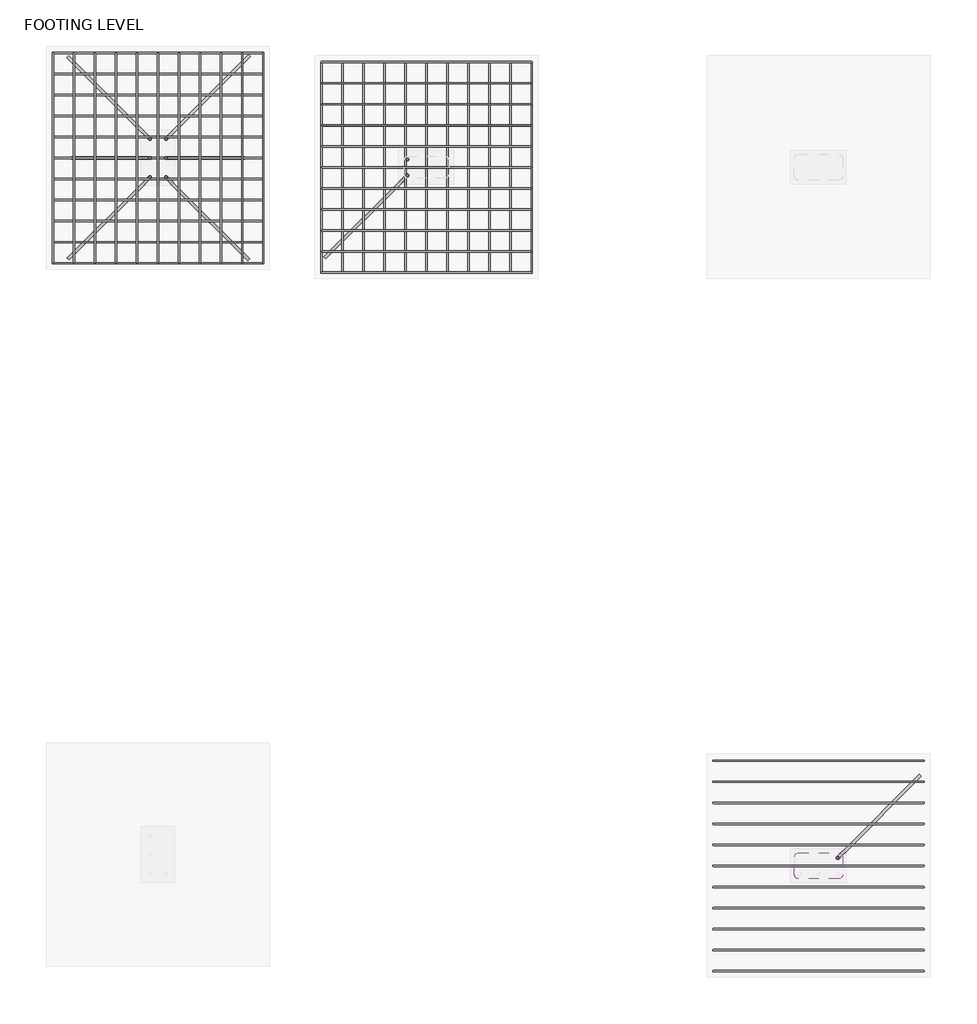
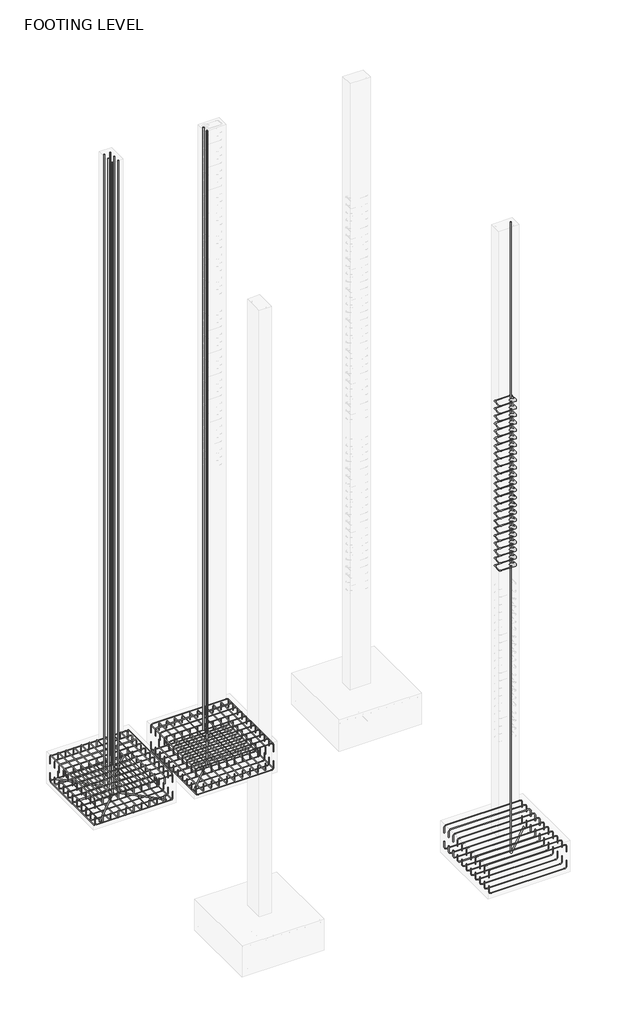
# One storey, part 3 of 10: 24 reinforcing bars.
"""IFC4 building model written with IfcOpenShell, lengths in millimetres."""

from ifc_helpers import new_model, si_unit, point, frame, origin, place, context, project, spatial, polyline, circle_curve, trimmed, segment, composite_curve, source, transform, mapped, element, save
from ifc_brep_helpers import swept_disk

model = new_model("IFC4")

# Units and contexts
model_context = context("Model", 3, world=origin())
ifc_project = project(units=[si_unit("LENGTHUNIT", "METRE", prefix="MILLI")], contexts=[model_context])

# Site, building, storey
site = spatial("IfcSite", under=ifc_project)
building = spatial("IfcBuilding", under=site)
storey = spatial("IfcBuildingStorey", under=building, Name="FOOTING LEVEL", Elevation=-1371.6)

# Reinforcing bars
placement = place(None, origin())
reinforcing_bar_shape = source(origin(), model_context, "Body", "SolidModel", [
    swept_disk(composite_curve([segment(polyline([(-12158.3043223, 4208.9876382, -1562.1), (-12158.3043223, 4208.9876382, -1447.8)]), True, "CONTINUOUS"), segment(trimmed(circle_curve(frame((-12191.6418223, 4208.9876382, -1447.8), z_axis=(0.0, -1.0, 0.0), x_axis=(33.337499999999636, 0.0, 0.0)), 33.3375), [point((-12158.3043223, 4208.9876382, -1447.8))], [point((-12191.6418223, 4208.9876382, -1414.4625))], True, "CARTESIAN"), True, "CONTINUOUS"), segment(polyline([(-12191.6418223, 4208.9876382, -1414.4625), (-13563.2418223, 4208.9876382, -1414.4625)]), True, "CONTINUOUS"), segment(trimmed(circle_curve(frame((-13563.2418223, 4208.9876382, -1447.8), z_axis=(0.0, -1.0, 0.0), x_axis=(0.0, 0.0, 33.337499999999864)), 33.3375), [point((-13563.2418223, 4208.9876382, -1414.4625))], [point((-13596.5793223, 4208.9876382, -1447.8))], True, "CARTESIAN"), True, "CONTINUOUS"), segment(polyline([(-13596.5793223, 4208.9876382, -1447.8), (-13596.5793223, 4208.9876382, -1562.1)]), True, "CONTINUOUS")], self_intersect=False), 4.7625),
])
element("IfcReinforcingBar", 1, at=placement, inside=storey, context=model_context, shape_type="MappedRepresentation", body=[
    mapped(reinforcing_bar_shape, transform((0.0, 0.0, 0.0), x_axis=(1.0, 0.0, 0.0), y_axis=(0.0, 1.0, 0.0), z_axis=(0.0, 0.0, 1.0))),
    mapped(reinforcing_bar_shape, transform((0.0, 143.8275, 0.0), x_axis=(1.0, 0.0, 0.0), y_axis=(0.0, 1.0, 0.0), z_axis=(0.0, 0.0, 1.0))),
    mapped(reinforcing_bar_shape, transform((0.0, 287.655, 0.0), x_axis=(1.0, 0.0, 0.0), y_axis=(0.0, 1.0, 0.0), z_axis=(0.0, 0.0, 1.0))),
    mapped(reinforcing_bar_shape, transform((0.0, 431.4825, 0.0), x_axis=(1.0, 0.0, 0.0), y_axis=(0.0, 1.0, 0.0), z_axis=(0.0, 0.0, 1.0))),
    mapped(reinforcing_bar_shape, transform((0.0, 575.31, 0.0), x_axis=(1.0, 0.0, 0.0), y_axis=(0.0, 1.0, 0.0), z_axis=(0.0, 0.0, 1.0))),
    mapped(reinforcing_bar_shape, transform((0.0, 719.1375, 0.0), x_axis=(1.0, 0.0, 0.0), y_axis=(0.0, 1.0, 0.0), z_axis=(0.0, 0.0, 1.0))),
    mapped(reinforcing_bar_shape, transform((0.0, 862.965, 0.0), x_axis=(1.0, 0.0, 0.0), y_axis=(0.0, 1.0, 0.0), z_axis=(0.0, 0.0, 1.0))),
    mapped(reinforcing_bar_shape, transform((0.0, 1006.7925, 0.0), x_axis=(1.0, 0.0, 0.0), y_axis=(0.0, 1.0, 0.0), z_axis=(0.0, 0.0, 1.0))),
    mapped(reinforcing_bar_shape, transform((0.0, 1150.62, 0.0), x_axis=(1.0, 0.0, 0.0), y_axis=(0.0, 1.0, 0.0), z_axis=(0.0, 0.0, 1.0))),
    mapped(reinforcing_bar_shape, transform((0.0, 1294.4475, 0.0), x_axis=(1.0, 0.0, 0.0), y_axis=(0.0, 1.0, 0.0), z_axis=(0.0, 0.0, 1.0))),
    mapped(reinforcing_bar_shape, transform((0.0, 1438.275, 0.0), x_axis=(1.0, 0.0, 0.0), y_axis=(0.0, 1.0, 0.0), z_axis=(0.0, 0.0, 1.0))),
])
reinforcing_bar_2_shape = source(origin(), model_context, "Body", "SolidModel", [
    swept_disk(composite_curve([segment(polyline([(-13596.5793223, 4208.9876382, -1790.7), (-13596.5793223, 4208.9876382, -1905.0)]), True, "CONTINUOUS"), segment(trimmed(circle_curve(frame((-13563.2418223, 4208.9876382, -1905.0), z_axis=(0.0, -1.0, 0.0), x_axis=(-33.337499999999636, 0.0, 0.0)), 33.3375), [point((-13596.5793223, 4208.9876382, -1905.0))], [point((-13563.2418223, 4208.9876382, -1938.3375))], True, "CARTESIAN"), True, "CONTINUOUS"), segment(polyline([(-13563.2418223, 4208.9876382, -1938.3375), (-12191.6418223, 4208.9876382, -1938.3375)]), True, "CONTINUOUS"), segment(trimmed(circle_curve(frame((-12191.6418223, 4208.9876382, -1905.0), z_axis=(0.0, -1.0, 0.0), x_axis=(0.0, 0.0, -33.33750000000009)), 33.3375), [point((-12191.6418223, 4208.9876382, -1938.3375))], [point((-12158.3043223, 4208.9876382, -1905.0))], True, "CARTESIAN"), True, "CONTINUOUS"), segment(polyline([(-12158.3043223, 4208.9876382, -1905.0), (-12158.3043223, 4208.9876382, -1790.7)]), True, "CONTINUOUS")], self_intersect=False), 4.7625),
])
element("IfcReinforcingBar", 2, at=placement, inside=storey, context=model_context, shape_type="MappedRepresentation", body=[
    mapped(reinforcing_bar_2_shape, transform((0.0, 0.0, 0.0), x_axis=(1.0, 0.0, 0.0), y_axis=(0.0, 1.0, 0.0), z_axis=(0.0, 0.0, 1.0))),
    mapped(reinforcing_bar_2_shape, transform((0.0, 143.8275, 0.0), x_axis=(1.0, 0.0, 0.0), y_axis=(0.0, 1.0, 0.0), z_axis=(0.0, 0.0, 1.0))),
    mapped(reinforcing_bar_2_shape, transform((0.0, 287.655, 0.0), x_axis=(1.0, 0.0, 0.0), y_axis=(0.0, 1.0, 0.0), z_axis=(0.0, 0.0, 1.0))),
    mapped(reinforcing_bar_2_shape, transform((0.0, 431.4825, 0.0), x_axis=(1.0, 0.0, 0.0), y_axis=(0.0, 1.0, 0.0), z_axis=(0.0, 0.0, 1.0))),
    mapped(reinforcing_bar_2_shape, transform((0.0, 575.31, 0.0), x_axis=(1.0, 0.0, 0.0), y_axis=(0.0, 1.0, 0.0), z_axis=(0.0, 0.0, 1.0))),
    mapped(reinforcing_bar_2_shape, transform((0.0, 719.1375, 0.0), x_axis=(1.0, 0.0, 0.0), y_axis=(0.0, 1.0, 0.0), z_axis=(0.0, 0.0, 1.0))),
    mapped(reinforcing_bar_2_shape, transform((0.0, 862.965, 0.0), x_axis=(1.0, 0.0, 0.0), y_axis=(0.0, 1.0, 0.0), z_axis=(0.0, 0.0, 1.0))),
    mapped(reinforcing_bar_2_shape, transform((0.0, 1006.7925, 0.0), x_axis=(1.0, 0.0, 0.0), y_axis=(0.0, 1.0, 0.0), z_axis=(0.0, 0.0, 1.0))),
    mapped(reinforcing_bar_2_shape, transform((0.0, 1150.62, 0.0), x_axis=(1.0, 0.0, 0.0), y_axis=(0.0, 1.0, 0.0), z_axis=(0.0, 0.0, 1.0))),
    mapped(reinforcing_bar_2_shape, transform((0.0, 1294.4475, 0.0), x_axis=(1.0, 0.0, 0.0), y_axis=(0.0, 1.0, 0.0), z_axis=(0.0, 0.0, 1.0))),
    mapped(reinforcing_bar_2_shape, transform((0.0, 1438.275, 0.0), x_axis=(1.0, 0.0, 0.0), y_axis=(0.0, 1.0, 0.0), z_axis=(0.0, 0.0, 1.0))),
])
reinforcing_bar_3_shape = source(origin(), model_context, "Body", "SolidModel", [
    swept_disk(composite_curve([segment(polyline([(-13596.5793223, 5647.2626382, -1770.864029), (-13596.5793223, 5647.2626382, -1885.164029)]), True, "CONTINUOUS"), segment(trimmed(circle_curve(frame((-13596.5793223, 5613.9251382, -1885.164029), z_axis=(-1.0, 0.0, 0.0), x_axis=(0.0, 33.337499999999636, 0.0)), 33.3375), [point((-13596.5793223, 5647.2626382, -1885.164029))], [point((-13596.5793223, 5613.9251382, -1918.501529))], True, "CARTESIAN"), True, "CONTINUOUS"), segment(polyline([(-13596.5793223, 5613.9251382, -1918.501529), (-13596.5793223, 4242.3251382, -1918.501529)]), True, "CONTINUOUS"), segment(trimmed(circle_curve(frame((-13596.5793223, 4242.3251382, -1885.164029), z_axis=(-1.0, 0.0, 0.0), x_axis=(0.0, 0.0, -33.337499999999864)), 33.3375), [point((-13596.5793223, 4242.3251382, -1918.501529))], [point((-13596.5793223, 4208.9876382, -1885.164029))], True, "CARTESIAN"), True, "CONTINUOUS"), segment(polyline([(-13596.5793223, 4208.9876382, -1885.164029), (-13596.5793223, 4208.9876382, -1770.864029)]), True, "CONTINUOUS")], self_intersect=False), 4.7625),
])
element("IfcReinforcingBar", 3, at=placement, inside=storey, context=model_context, shape_type="MappedRepresentation", body=[
    mapped(reinforcing_bar_3_shape, transform((0.0, 0.0, 0.0), x_axis=(1.0, 0.0, 0.0), y_axis=(0.0, 1.0, 0.0), z_axis=(0.0, 0.0, 1.0))),
    mapped(reinforcing_bar_3_shape, transform((143.8275, 0.0, 0.0), x_axis=(1.0, 0.0, 0.0), y_axis=(0.0, 1.0, 0.0), z_axis=(0.0, 0.0, 1.0))),
    mapped(reinforcing_bar_3_shape, transform((287.655, 0.0, 0.0), x_axis=(1.0, 0.0, 0.0), y_axis=(0.0, 1.0, 0.0), z_axis=(0.0, 0.0, 1.0))),
    mapped(reinforcing_bar_3_shape, transform((431.4825, 0.0, 0.0), x_axis=(1.0, 0.0, 0.0), y_axis=(0.0, 1.0, 0.0), z_axis=(0.0, 0.0, 1.0))),
    mapped(reinforcing_bar_3_shape, transform((575.31, 0.0, 0.0), x_axis=(1.0, 0.0, 0.0), y_axis=(0.0, 1.0, 0.0), z_axis=(0.0, 0.0, 1.0))),
    mapped(reinforcing_bar_3_shape, transform((719.1375, 0.0, 0.0), x_axis=(1.0, 0.0, 0.0), y_axis=(0.0, 1.0, 0.0), z_axis=(0.0, 0.0, 1.0))),
    mapped(reinforcing_bar_3_shape, transform((862.965, 0.0, 0.0), x_axis=(1.0, 0.0, 0.0), y_axis=(0.0, 1.0, 0.0), z_axis=(0.0, 0.0, 1.0))),
    mapped(reinforcing_bar_3_shape, transform((1006.7925, 0.0, 0.0), x_axis=(1.0, 0.0, 0.0), y_axis=(0.0, 1.0, 0.0), z_axis=(0.0, 0.0, 1.0))),
    mapped(reinforcing_bar_3_shape, transform((1150.62, 0.0, 0.0), x_axis=(1.0, 0.0, 0.0), y_axis=(0.0, 1.0, 0.0), z_axis=(0.0, 0.0, 1.0))),
    mapped(reinforcing_bar_3_shape, transform((1294.4475, 0.0, 0.0), x_axis=(1.0, 0.0, 0.0), y_axis=(0.0, 1.0, 0.0), z_axis=(0.0, 0.0, 1.0))),
    mapped(reinforcing_bar_3_shape, transform((1438.275, 0.0, 0.0), x_axis=(1.0, 0.0, 0.0), y_axis=(0.0, 1.0, 0.0), z_axis=(0.0, 0.0, 1.0))),
])
reinforcing_bar_4_shape = source(origin(), model_context, "Body", "SolidModel", [
    swept_disk(composite_curve([segment(polyline([(-12158.3043223, 5647.2626382, -1586.5406765), (-12158.3043223, 5647.2626382, -1472.2406765)]), True, "CONTINUOUS"), segment(trimmed(circle_curve(frame((-12158.3043223, 5613.9251382, -1472.2406765), z_axis=(1.0, 0.0, 0.0), x_axis=(0.0, 33.337499999999636, 0.0)), 33.3375), [point((-12158.3043223, 5647.2626382, -1472.2406765))], [point((-12158.3043223, 5613.9251382, -1438.9031765))], True, "CARTESIAN"), True, "CONTINUOUS"), segment(polyline([(-12158.3043223, 5613.9251382, -1438.9031765), (-12158.3043223, 4242.3251382, -1438.9031765)]), True, "CONTINUOUS"), segment(trimmed(circle_curve(frame((-12158.3043223, 4242.3251382, -1472.2406765), z_axis=(1.0, 0.0, 0.0), x_axis=(0.0, 0.0, 33.33750000000009)), 33.3375), [point((-12158.3043223, 4242.3251382, -1438.9031765))], [point((-12158.3043223, 4208.9876382, -1472.2406765))], True, "CARTESIAN"), True, "CONTINUOUS"), segment(polyline([(-12158.3043223, 4208.9876382, -1472.2406765), (-12158.3043223, 4208.9876382, -1586.5406765)]), True, "CONTINUOUS")], self_intersect=False), 4.7625),
])
element("IfcReinforcingBar", 4, at=placement, inside=storey, context=model_context, shape_type="MappedRepresentation", body=[
    mapped(reinforcing_bar_4_shape, transform((0.0, 0.0, 0.0), x_axis=(1.0, 0.0, 0.0), y_axis=(0.0, 1.0, 0.0), z_axis=(0.0, 0.0, 1.0))),
    mapped(reinforcing_bar_4_shape, transform((-143.8275, 0.0, 0.0), x_axis=(1.0, 0.0, 0.0), y_axis=(0.0, 1.0, 0.0), z_axis=(0.0, 0.0, 1.0))),
    mapped(reinforcing_bar_4_shape, transform((-287.655, 0.0, 0.0), x_axis=(1.0, 0.0, 0.0), y_axis=(0.0, 1.0, 0.0), z_axis=(0.0, 0.0, 1.0))),
    mapped(reinforcing_bar_4_shape, transform((-431.4825, 0.0, 0.0), x_axis=(1.0, 0.0, 0.0), y_axis=(0.0, 1.0, 0.0), z_axis=(0.0, 0.0, 1.0))),
    mapped(reinforcing_bar_4_shape, transform((-575.31, 0.0, 0.0), x_axis=(1.0, 0.0, 0.0), y_axis=(0.0, 1.0, 0.0), z_axis=(0.0, 0.0, 1.0))),
    mapped(reinforcing_bar_4_shape, transform((-719.1375, 0.0, 0.0), x_axis=(1.0, 0.0, 0.0), y_axis=(0.0, 1.0, 0.0), z_axis=(0.0, 0.0, 1.0))),
    mapped(reinforcing_bar_4_shape, transform((-862.965, 0.0, 0.0), x_axis=(1.0, 0.0, 0.0), y_axis=(0.0, 1.0, 0.0), z_axis=(0.0, 0.0, 1.0))),
    mapped(reinforcing_bar_4_shape, transform((-1006.7925, 0.0, 0.0), x_axis=(1.0, 0.0, 0.0), y_axis=(0.0, 1.0, 0.0), z_axis=(0.0, 0.0, 1.0))),
    mapped(reinforcing_bar_4_shape, transform((-1150.62, 0.0, 0.0), x_axis=(1.0, 0.0, 0.0), y_axis=(0.0, 1.0, 0.0), z_axis=(0.0, 0.0, 1.0))),
    mapped(reinforcing_bar_4_shape, transform((-1294.4475, 0.0, 0.0), x_axis=(1.0, 0.0, 0.0), y_axis=(0.0, 1.0, 0.0), z_axis=(0.0, 0.0, 1.0))),
    mapped(reinforcing_bar_4_shape, transform((-1438.275, 0.0, 0.0), x_axis=(1.0, 0.0, 0.0), y_axis=(0.0, 1.0, 0.0), z_axis=(0.0, 0.0, 1.0))),
])
reinforcing_bar_5_shape = source(origin(), model_context, "Body", "SolidModel", [
    swept_disk(composite_curve([segment(polyline([(-13993.4543223, 5711.1953802, -1562.1), (-13993.4543223, 5711.1953802, -1447.8)]), True, "CONTINUOUS"), segment(trimmed(circle_curve(frame((-13993.4543223, 5677.8578802, -1447.8), z_axis=(1.0, 0.0, 0.0), x_axis=(0.0, 33.337499999999636, 0.0)), 33.3375), [point((-13993.4543223, 5711.1953802, -1447.8))], [point((-13993.4543223, 5677.8578802, -1414.4625))], True, "CARTESIAN"), True, "CONTINUOUS"), segment(polyline([(-13993.4543223, 5677.8578802, -1414.4625), (-13993.4543223, 4306.2578802, -1414.4625)]), True, "CONTINUOUS"), segment(trimmed(circle_curve(frame((-13993.4543223, 4306.2578802, -1447.8), z_axis=(1.0, 0.0, 0.0), x_axis=(0.0, 0.0, 33.337499999999864)), 33.3375), [point((-13993.4543223, 4306.2578802, -1414.4625))], [point((-13993.4543223, 4272.9203802, -1447.8))], True, "CARTESIAN"), True, "CONTINUOUS"), segment(polyline([(-13993.4543223, 4272.9203802, -1447.8), (-13993.4543223, 4272.9203802, -1562.1)]), True, "CONTINUOUS")], self_intersect=False), 4.7625),
])
element("IfcReinforcingBar", 5, at=placement, inside=storey, context=model_context, shape_type="MappedRepresentation", body=[
    mapped(reinforcing_bar_5_shape, transform((0.0, 0.0, 0.0), x_axis=(1.0, 0.0, 0.0), y_axis=(0.0, 1.0, 0.0), z_axis=(0.0, 0.0, 1.0))),
    mapped(reinforcing_bar_5_shape, transform((-143.8275, 0.0, 0.0), x_axis=(1.0, 0.0, 0.0), y_axis=(0.0, 1.0, 0.0), z_axis=(0.0, 0.0, 1.0))),
    mapped(reinforcing_bar_5_shape, transform((-287.655, 0.0, 0.0), x_axis=(1.0, 0.0, 0.0), y_axis=(0.0, 1.0, 0.0), z_axis=(0.0, 0.0, 1.0))),
    mapped(reinforcing_bar_5_shape, transform((-431.4825, 0.0, 0.0), x_axis=(1.0, 0.0, 0.0), y_axis=(0.0, 1.0, 0.0), z_axis=(0.0, 0.0, 1.0))),
    mapped(reinforcing_bar_5_shape, transform((-575.31, 0.0, 0.0), x_axis=(1.0, 0.0, 0.0), y_axis=(0.0, 1.0, 0.0), z_axis=(0.0, 0.0, 1.0))),
    mapped(reinforcing_bar_5_shape, transform((-719.1375, 0.0, 0.0), x_axis=(1.0, 0.0, 0.0), y_axis=(0.0, 1.0, 0.0), z_axis=(0.0, 0.0, 1.0))),
    mapped(reinforcing_bar_5_shape, transform((-862.965, 0.0, 0.0), x_axis=(1.0, 0.0, 0.0), y_axis=(0.0, 1.0, 0.0), z_axis=(0.0, 0.0, 1.0))),
    mapped(reinforcing_bar_5_shape, transform((-1006.7925, 0.0, 0.0), x_axis=(1.0, 0.0, 0.0), y_axis=(0.0, 1.0, 0.0), z_axis=(0.0, 0.0, 1.0))),
    mapped(reinforcing_bar_5_shape, transform((-1150.62, 0.0, 0.0), x_axis=(1.0, 0.0, 0.0), y_axis=(0.0, 1.0, 0.0), z_axis=(0.0, 0.0, 1.0))),
    mapped(reinforcing_bar_5_shape, transform((-1294.4475, 0.0, 0.0), x_axis=(1.0, 0.0, 0.0), y_axis=(0.0, 1.0, 0.0), z_axis=(0.0, 0.0, 1.0))),
    mapped(reinforcing_bar_5_shape, transform((-1438.275, 0.0, 0.0), x_axis=(1.0, 0.0, 0.0), y_axis=(0.0, 1.0, 0.0), z_axis=(0.0, 0.0, 1.0))),
])
reinforcing_bar_6_shape = source(origin(), model_context, "Body", "SolidModel", [
    swept_disk(composite_curve([segment(polyline([(-13993.4543223, 4272.9203802, -1790.7), (-13993.4543223, 4272.9203802, -1905.0)]), True, "CONTINUOUS"), segment(trimmed(circle_curve(frame((-13993.4543223, 4306.2578802, -1905.0), z_axis=(1.0, 0.0, 0.0), x_axis=(0.0, -33.337499999999636, 0.0)), 33.3375), [point((-13993.4543223, 4272.9203802, -1905.0))], [point((-13993.4543223, 4306.2578802, -1938.3375))], True, "CARTESIAN"), True, "CONTINUOUS"), segment(polyline([(-13993.4543223, 4306.2578802, -1938.3375), (-13993.4543223, 5677.8578802, -1938.3375)]), True, "CONTINUOUS"), segment(trimmed(circle_curve(frame((-13993.4543223, 5677.8578802, -1905.0), z_axis=(1.0, 0.0, 0.0), x_axis=(0.0, 0.0, -33.33750000000009)), 33.3375), [point((-13993.4543223, 5677.8578802, -1938.3375))], [point((-13993.4543223, 5711.1953802, -1905.0))], True, "CARTESIAN"), True, "CONTINUOUS"), segment(polyline([(-13993.4543223, 5711.1953802, -1905.0), (-13993.4543223, 5711.1953802, -1790.7)]), True, "CONTINUOUS")], self_intersect=False), 4.7625),
])
element("IfcReinforcingBar", 6, at=placement, inside=storey, context=model_context, shape_type="MappedRepresentation", body=[
    mapped(reinforcing_bar_6_shape, transform((0.0, 0.0, 0.0), x_axis=(1.0, 0.0, 0.0), y_axis=(0.0, 1.0, 0.0), z_axis=(0.0, 0.0, 1.0))),
    mapped(reinforcing_bar_6_shape, transform((-143.8275, 0.0, 0.0), x_axis=(1.0, 0.0, 0.0), y_axis=(0.0, 1.0, 0.0), z_axis=(0.0, 0.0, 1.0))),
    mapped(reinforcing_bar_6_shape, transform((-287.655, 0.0, 0.0), x_axis=(1.0, 0.0, 0.0), y_axis=(0.0, 1.0, 0.0), z_axis=(0.0, 0.0, 1.0))),
    mapped(reinforcing_bar_6_shape, transform((-431.4825, 0.0, 0.0), x_axis=(1.0, 0.0, 0.0), y_axis=(0.0, 1.0, 0.0), z_axis=(0.0, 0.0, 1.0))),
    mapped(reinforcing_bar_6_shape, transform((-575.31, 0.0, 0.0), x_axis=(1.0, 0.0, 0.0), y_axis=(0.0, 1.0, 0.0), z_axis=(0.0, 0.0, 1.0))),
    mapped(reinforcing_bar_6_shape, transform((-719.1375, 0.0, 0.0), x_axis=(1.0, 0.0, 0.0), y_axis=(0.0, 1.0, 0.0), z_axis=(0.0, 0.0, 1.0))),
    mapped(reinforcing_bar_6_shape, transform((-862.965, 0.0, 0.0), x_axis=(1.0, 0.0, 0.0), y_axis=(0.0, 1.0, 0.0), z_axis=(0.0, 0.0, 1.0))),
    mapped(reinforcing_bar_6_shape, transform((-1006.7925, 0.0, 0.0), x_axis=(1.0, 0.0, 0.0), y_axis=(0.0, 1.0, 0.0), z_axis=(0.0, 0.0, 1.0))),
    mapped(reinforcing_bar_6_shape, transform((-1150.62, 0.0, 0.0), x_axis=(1.0, 0.0, 0.0), y_axis=(0.0, 1.0, 0.0), z_axis=(0.0, 0.0, 1.0))),
    mapped(reinforcing_bar_6_shape, transform((-1294.4475, 0.0, 0.0), x_axis=(1.0, 0.0, 0.0), y_axis=(0.0, 1.0, 0.0), z_axis=(0.0, 0.0, 1.0))),
    mapped(reinforcing_bar_6_shape, transform((-1438.275, 0.0, 0.0), x_axis=(1.0, 0.0, 0.0), y_axis=(0.0, 1.0, 0.0), z_axis=(0.0, 0.0, 1.0))),
])
reinforcing_bar_7_shape = source(origin(), model_context, "Body", "SolidModel", [
    swept_disk(composite_curve([segment(polyline([(-15431.7293223, 4272.9203802, -1770.864029), (-15431.7293223, 4272.9203802, -1885.164029)]), True, "CONTINUOUS"), segment(trimmed(circle_curve(frame((-15398.3918223, 4272.9203802, -1885.164029), z_axis=(0.0, -1.0, 0.0), x_axis=(-33.337499999999636, 0.0, 0.0)), 33.3375), [point((-15431.7293223, 4272.9203802, -1885.164029))], [point((-15398.3918223, 4272.9203802, -1918.501529))], True, "CARTESIAN"), True, "CONTINUOUS"), segment(polyline([(-15398.3918223, 4272.9203802, -1918.501529), (-14026.7918223, 4272.9203802, -1918.501529)]), True, "CONTINUOUS"), segment(trimmed(circle_curve(frame((-14026.7918223, 4272.9203802, -1885.164029), z_axis=(0.0, -1.0, 0.0), x_axis=(0.0, 0.0, -33.337499999999864)), 33.3375), [point((-14026.7918223, 4272.9203802, -1918.501529))], [point((-13993.4543223, 4272.9203802, -1885.164029))], True, "CARTESIAN"), True, "CONTINUOUS"), segment(polyline([(-13993.4543223, 4272.9203802, -1885.164029), (-13993.4543223, 4272.9203802, -1770.864029)]), True, "CONTINUOUS")], self_intersect=False), 4.7625),
])
element("IfcReinforcingBar", 7, at=placement, inside=storey, context=model_context, shape_type="MappedRepresentation", body=[
    mapped(reinforcing_bar_7_shape, transform((0.0, 0.0, 0.0), x_axis=(1.0, 0.0, 0.0), y_axis=(0.0, 1.0, 0.0), z_axis=(0.0, 0.0, 1.0))),
    mapped(reinforcing_bar_7_shape, transform((0.0, 143.8275, 0.0), x_axis=(1.0, 0.0, 0.0), y_axis=(0.0, 1.0, 0.0), z_axis=(0.0, 0.0, 1.0))),
    mapped(reinforcing_bar_7_shape, transform((0.0, 287.655, 0.0), x_axis=(1.0, 0.0, 0.0), y_axis=(0.0, 1.0, 0.0), z_axis=(0.0, 0.0, 1.0))),
    mapped(reinforcing_bar_7_shape, transform((0.0, 431.4825, 0.0), x_axis=(1.0, 0.0, 0.0), y_axis=(0.0, 1.0, 0.0), z_axis=(0.0, 0.0, 1.0))),
    mapped(reinforcing_bar_7_shape, transform((0.0, 575.31, 0.0), x_axis=(1.0, 0.0, 0.0), y_axis=(0.0, 1.0, 0.0), z_axis=(0.0, 0.0, 1.0))),
    mapped(reinforcing_bar_7_shape, transform((0.0, 719.1375, 0.0), x_axis=(1.0, 0.0, 0.0), y_axis=(0.0, 1.0, 0.0), z_axis=(0.0, 0.0, 1.0))),
    mapped(reinforcing_bar_7_shape, transform((0.0, 862.965, 0.0), x_axis=(1.0, 0.0, 0.0), y_axis=(0.0, 1.0, 0.0), z_axis=(0.0, 0.0, 1.0))),
    mapped(reinforcing_bar_7_shape, transform((0.0, 1006.7925, 0.0), x_axis=(1.0, 0.0, 0.0), y_axis=(0.0, 1.0, 0.0), z_axis=(0.0, 0.0, 1.0))),
    mapped(reinforcing_bar_7_shape, transform((0.0, 1150.62, 0.0), x_axis=(1.0, 0.0, 0.0), y_axis=(0.0, 1.0, 0.0), z_axis=(0.0, 0.0, 1.0))),
    mapped(reinforcing_bar_7_shape, transform((0.0, 1294.4475, 0.0), x_axis=(1.0, 0.0, 0.0), y_axis=(0.0, 1.0, 0.0), z_axis=(0.0, 0.0, 1.0))),
    mapped(reinforcing_bar_7_shape, transform((0.0, 1438.275, 0.0), x_axis=(1.0, 0.0, 0.0), y_axis=(0.0, 1.0, 0.0), z_axis=(0.0, 0.0, 1.0))),
])
reinforcing_bar_8_shape = source(origin(), model_context, "Body", "SolidModel", [
    swept_disk(composite_curve([segment(polyline([(-15431.7293223, 5711.1953802, -1586.5406765), (-15431.7293223, 5711.1953802, -1472.2406765)]), True, "CONTINUOUS"), segment(trimmed(circle_curve(frame((-15398.3918223, 5711.1953802, -1472.2406765), z_axis=(0.0, 1.0, 0.0), x_axis=(-33.337499999999636, 0.0, 0.0)), 33.3375), [point((-15431.7293223, 5711.1953802, -1472.2406765))], [point((-15398.3918223, 5711.1953802, -1438.9031765))], True, "CARTESIAN"), True, "CONTINUOUS"), segment(polyline([(-15398.3918223, 5711.1953802, -1438.9031765), (-14026.7918223, 5711.1953802, -1438.9031765)]), True, "CONTINUOUS"), segment(trimmed(circle_curve(frame((-14026.7918223, 5711.1953802, -1472.2406765), z_axis=(0.0, 1.0, 0.0), x_axis=(0.0, 0.0, 33.33750000000009)), 33.3375), [point((-14026.7918223, 5711.1953802, -1438.9031765))], [point((-13993.4543223, 5711.1953802, -1472.2406765))], True, "CARTESIAN"), True, "CONTINUOUS"), segment(polyline([(-13993.4543223, 5711.1953802, -1472.2406765), (-13993.4543223, 5711.1953802, -1586.5406765)]), True, "CONTINUOUS")], self_intersect=False), 4.7625),
])
element("IfcReinforcingBar", 8, at=placement, inside=storey, context=model_context, shape_type="MappedRepresentation", body=[
    mapped(reinforcing_bar_8_shape, transform((0.0, 0.0, 0.0), x_axis=(1.0, 0.0, 0.0), y_axis=(0.0, 1.0, 0.0), z_axis=(0.0, 0.0, 1.0))),
    mapped(reinforcing_bar_8_shape, transform((0.0, -143.8275, 0.0), x_axis=(1.0, 0.0, 0.0), y_axis=(0.0, 1.0, 0.0), z_axis=(0.0, 0.0, 1.0))),
    mapped(reinforcing_bar_8_shape, transform((0.0, -287.655, 0.0), x_axis=(1.0, 0.0, 0.0), y_axis=(0.0, 1.0, 0.0), z_axis=(0.0, 0.0, 1.0))),
    mapped(reinforcing_bar_8_shape, transform((0.0, -431.4825, 0.0), x_axis=(1.0, 0.0, 0.0), y_axis=(0.0, 1.0, 0.0), z_axis=(0.0, 0.0, 1.0))),
    mapped(reinforcing_bar_8_shape, transform((0.0, -575.31, 0.0), x_axis=(1.0, 0.0, 0.0), y_axis=(0.0, 1.0, 0.0), z_axis=(0.0, 0.0, 1.0))),
    mapped(reinforcing_bar_8_shape, transform((0.0, -719.1375, 0.0), x_axis=(1.0, 0.0, 0.0), y_axis=(0.0, 1.0, 0.0), z_axis=(0.0, 0.0, 1.0))),
    mapped(reinforcing_bar_8_shape, transform((0.0, -862.965, 0.0), x_axis=(1.0, 0.0, 0.0), y_axis=(0.0, 1.0, 0.0), z_axis=(0.0, 0.0, 1.0))),
    mapped(reinforcing_bar_8_shape, transform((0.0, -1006.7925, 0.0), x_axis=(1.0, 0.0, 0.0), y_axis=(0.0, 1.0, 0.0), z_axis=(0.0, 0.0, 1.0))),
    mapped(reinforcing_bar_8_shape, transform((0.0, -1150.62, 0.0), x_axis=(1.0, 0.0, 0.0), y_axis=(0.0, 1.0, 0.0), z_axis=(0.0, 0.0, 1.0))),
    mapped(reinforcing_bar_8_shape, transform((0.0, -1294.4475, 0.0), x_axis=(1.0, 0.0, 0.0), y_axis=(0.0, 1.0, 0.0), z_axis=(0.0, 0.0, 1.0))),
    mapped(reinforcing_bar_8_shape, transform((0.0, -1438.275, 0.0), x_axis=(1.0, 0.0, 0.0), y_axis=(0.0, 1.0, 0.0), z_axis=(0.0, 0.0, 1.0))),
])
element("IfcReinforcingBar", 9, at=placement, inside=storey, context=model_context, shape_type="SolidModel", body=[
    swept_disk(composite_curve([segment(polyline([(-9503.0028099, 771.8966837, -1910.4342608), (-10020.0352856, 254.864208, -1910.4342608)]), True, "CONTINUOUS"), segment(trimmed(circle_curve(frame((-10020.0352856, 254.864208, -1843.7592608), z_axis=(-0.7071067811865249, 0.7071067811865701, 0.0), x_axis=(0.0, 0.0, -66.67499999999995)), 66.675), [point((-10020.0352856, 254.864208, -1910.4342608))], [point((-10067.1816302, 207.7178633, -1843.7592608))], True, "CARTESIAN"), True, "CONTINUOUS"), segment(polyline([(-10067.1816302, 207.7178633, -1843.7592608), (-10067.1816302, 207.7178633, 10490.2)]), True, "CONTINUOUS")], self_intersect=False), 9.525),
])
element("IfcReinforcingBar", 10, at=placement, inside=storey, context=model_context, shape_type="SolidModel", body=[
    swept_disk(composite_curve([segment(polyline([(-14658.2316302, 5122.6180723, -1333.5), (-14658.2316302, 5122.6180723, 10477.5)]), True, "CONTINUOUS")], self_intersect=False), 9.525),
])
element("IfcReinforcingBar", 11, at=placement, inside=storey, context=model_context, shape_type="SolidModel", body=[
    swept_disk(composite_curve([segment(polyline([(-14766.9520144, 4861.4976881, -1333.5), (-14766.9520144, 4861.4976881, 10477.5)]), True, "CONTINUOUS")], self_intersect=False), 9.525),
])
element("IfcReinforcingBar", 12, at=placement, inside=storey, context=model_context, shape_type="SolidModel", body=[
    swept_disk(composite_curve([segment(polyline([(-14658.2316302, 4861.4976881, -1333.5), (-14658.2316302, 4861.4976881, 10477.5)]), True, "CONTINUOUS")], self_intersect=False), 9.525),
])
element("IfcReinforcingBar", 13, at=placement, inside=storey, context=model_context, shape_type="SolidModel", body=[
    swept_disk(composite_curve([segment(polyline([(-15328.6277703, 5684.2938282, -1910.4342608), (-14814.0983591, 5169.7644169, -1910.4342608)]), True, "CONTINUOUS"), segment(trimmed(circle_curve(frame((-14814.0983591, 5169.7644169, -1843.7592608), z_axis=(-0.7071067811865737, -0.7071067811865215, 0.0), x_axis=(0.0, 0.0, -66.67499999999995)), 66.675), [point((-14814.0983591, 5169.7644169, -1910.4342608))], [point((-14766.9520144, 5122.6180723, -1843.7592608))], True, "CARTESIAN"), True, "CONTINUOUS"), segment(polyline([(-14766.9520144, 5122.6180723, -1843.7592608), (-14766.9520144, 5122.6180723, 10477.5)]), True, "CONTINUOUS")], self_intersect=False), 9.525),
])
element("IfcReinforcingBar", 14, at=placement, inside=storey, context=model_context, shape_type="SolidModel", body=[
    swept_disk(composite_curve([segment(polyline([(-14088.5374965, 5692.312206, -1910.4342608), (-14611.0852856, 5169.7644169, -1910.4342608)]), True, "CONTINUOUS"), segment(trimmed(circle_curve(frame((-14611.0852856, 5169.7644169, -1843.7592608), z_axis=(-0.7071067811865711, 0.7071067811865239, 0.0), x_axis=(0.0, 0.0, -66.67499999999995)), 66.675), [point((-14611.0852856, 5169.7644169, -1910.4342608))], [point((-14658.2316302, 5122.6180723, -1843.7592608))], True, "CARTESIAN"), True, "CONTINUOUS"), segment(polyline([(-14658.2316302, 5122.6180723, -1843.7592608), (-14658.2316302, 5122.6180723, 10477.5)]), True, "CONTINUOUS")], self_intersect=False), 9.525),
])
element("IfcReinforcingBar", 15, at=placement, inside=storey, context=model_context, shape_type="SolidModel", body=[
    swept_disk(composite_curve([segment(polyline([(-15325.6711349, 4302.7785676, -1910.4342608), (-14814.0983591, 4814.3513434, -1910.4342608)]), True, "CONTINUOUS"), segment(trimmed(circle_curve(frame((-14814.0983591, 4814.3513434, -1843.7592608), z_axis=(0.7071067811865759, -0.7071067811865193, 0.0), x_axis=(0.0, 0.0, -66.67499999999995)), 66.675), [point((-14814.0983591, 4814.3513434, -1910.4342608))], [point((-14766.9520144, 4861.4976881, -1843.7592608))], True, "CARTESIAN"), True, "CONTINUOUS"), segment(polyline([(-14766.9520144, 4861.4976881, -1843.7592608), (-14766.9520144, 4861.4976881, 10477.5)]), True, "CONTINUOUS")], self_intersect=False), 9.525),
])
element("IfcReinforcingBar", 16, at=placement, inside=storey, context=model_context, shape_type="SolidModel", body=[
    swept_disk(composite_curve([segment(polyline([(-14094.0528099, 4297.3188678, -1910.4342608), (-14611.0852856, 4814.3513434, -1910.4342608)]), True, "CONTINUOUS"), segment(trimmed(circle_curve(frame((-14611.0852856, 4814.3513434, -1843.7592608), z_axis=(0.707106781186569, 0.707106781186526, 0.0), x_axis=(0.0, 0.0, -66.67499999999995)), 66.675), [point((-14611.0852856, 4814.3513434, -1910.4342608))], [point((-14658.2316302, 4861.4976881, -1843.7592608))], True, "CARTESIAN"), True, "CONTINUOUS"), segment(polyline([(-14658.2316302, 4861.4976881, -1843.7592608), (-14658.2316302, 4861.4976881, 10477.5)]), True, "CONTINUOUS")], self_intersect=False), 9.525),
])
element("IfcReinforcingBar", 17, at=placement, inside=storey, context=model_context, shape_type="SolidModel", body=[
    swept_disk(composite_curve([segment(polyline([(-15305.1818909, 4992.0578802, -1910.4342608), (-14833.6270144, 4992.0578802, -1910.4342608)]), True, "CONTINUOUS"), segment(trimmed(circle_curve(frame((-14833.6270144, 4992.0578802, -1843.7592608), z_axis=(0.0, -1.0, 0.0), x_axis=(0.0, 0.0, -66.67499999999995)), 66.675), [point((-14833.6270144, 4992.0578802, -1910.4342608))], [point((-14766.9520144, 4992.0578802, -1843.7592608))], True, "CARTESIAN"), True, "CONTINUOUS"), segment(polyline([(-14766.9520144, 4992.0578802, -1843.7592608), (-14766.9520144, 4992.0578802, 10477.5)]), True, "CONTINUOUS")], self_intersect=False), 9.525),
])
element("IfcReinforcingBar", 18, at=placement, inside=storey, context=model_context, shape_type="SolidModel", body=[
    swept_disk(composite_curve([segment(polyline([(-13008.0020144, 4982.4853303, -1333.5), (-13008.0020144, 4982.4853303, 10477.5)]), True, "CONTINUOUS")], self_intersect=False), 9.525),
])
element("IfcReinforcingBar", 19, at=placement, inside=storey, context=model_context, shape_type="SolidModel", body=[
    swept_disk(composite_curve([segment(polyline([(-13008.0020144, 4873.7649461, -1333.5), (-13008.0020144, 4873.7649461, 10477.5)]), True, "CONTINUOUS")], self_intersect=False), 9.525),
])
element("IfcReinforcingBar", 20, at=placement, inside=storey, context=model_context, shape_type="SolidModel", body=[
    swept_disk(composite_curve([segment(polyline([(-13572.1808347, 4309.5861258, -1910.4342608), (-13055.1483591, 4826.6186014, -1910.4342608)]), True, "CONTINUOUS"), segment(trimmed(circle_curve(frame((-13055.1483591, 4826.6186014, -1843.7592608), z_axis=(0.707106781186523, -0.707106781186572, 0.0), x_axis=(0.0, 0.0, -66.67499999999995)), 66.675), [point((-13055.1483591, 4826.6186014, -1910.4342608))], [point((-13008.0020144, 4873.7649461, -1843.7592608))], True, "CARTESIAN"), True, "CONTINUOUS"), segment(polyline([(-13008.0020144, 4873.7649461, -1843.7592608), (-13008.0020144, 4873.7649461, 10477.5)]), True, "CONTINUOUS")], self_intersect=False), 9.525),
])
element("IfcReinforcingBar", 21, at=placement, inside=storey, context=model_context, shape_type="SolidModel", body=[
    swept_disk(composite_curve([segment(polyline([(-14120.0017538, 4992.0578802, -1910.4342608), (-14591.5566302, 4992.0578802, -1910.4342608)]), True, "CONTINUOUS"), segment(trimmed(circle_curve(frame((-14591.5566302, 4992.0578802, -1843.7592608), z_axis=(0.0, 1.0, 0.0), x_axis=(0.0, 0.0, -66.67499999999995)), 66.675), [point((-14591.5566302, 4992.0578802, -1910.4342608))], [point((-14658.2316302, 4992.0578802, -1843.7592608))], True, "CARTESIAN"), True, "CONTINUOUS"), segment(polyline([(-14658.2316302, 4992.0578802, -1843.7592608), (-14658.2316302, 4992.0578802, 10477.5)]), True, "CONTINUOUS")], self_intersect=False), 9.525),
])
reinforcing_bar_9_shape = source(origin(), model_context, "Body", "SolidModel", [
    swept_disk(composite_curve([segment(polyline([(-10134.9189996, 133.0588881, 3840.1625), (-10078.0548026, 76.194691, 3840.1625)]), True, "CONTINUOUS"), segment(trimmed(circle_curve(frame((-10061.2168223, 93.0326713, 3840.1625), z_axis=(0.0, 0.0, 1.0), x_axis=(-16.83798029999889, -16.837980299999998, 0.0)), 23.8125), [point((-10078.0548026, 76.194691, 3840.1625))], [point((-10037.4043223, 93.0326713, 3840.1625))], True, "CARTESIAN"), True, "CONTINUOUS"), segment(polyline([(-10037.4043223, 93.0326713, 3840.1625), (-10037.4043223, 213.6826713, 3840.1625)]), True, "CONTINUOUS"), segment(trimmed(circle_curve(frame((-10061.2168223, 213.6826713, 3840.1625), z_axis=(0.0, 0.0, 1.0), x_axis=(23.8125, 0.0, 0.0)), 23.8125), [point((-10037.4043223, 213.6826713, 3840.1625))], [point((-10061.2168223, 237.4951713, 3840.1625))], True, "CARTESIAN"), True, "CONTINUOUS"), segment(polyline([(-10061.2168223, 237.4951713, 3840.1625), (-10334.2668223, 237.4951713, 3840.1625)]), True, "CONTINUOUS"), segment(trimmed(circle_curve(frame((-10334.2668223, 213.7207273, 3838.8167768), z_axis=(0.0, -0.056513312022655804, 0.9984018457335854), x_axis=(0.0, 23.774444000000017, 1.3457232000000658)), 23.8125), [point((-10334.2668223, 237.4951713, 3840.1625))], [point((-10358.0793223, 213.7207273, 3838.8167768))], True, "CARTESIAN"), True, "CONTINUOUS"), segment(polyline([(-10358.0793223, 213.7207273, 3838.8167768), (-10358.0793223, 92.9946152, 3831.9832232)]), True, "CONTINUOUS"), segment(trimmed(circle_curve(frame((-10334.2668223, 92.9946152, 3831.9832232), z_axis=(0.0, -0.056513312022655804, 0.9984018457335854), x_axis=(-23.8125, 0.0, 0.0)), 23.8125), [point((-10358.0793223, 92.9946152, 3831.9832232))], [point((-10334.2668223, 69.2201713, 3830.6375))], True, "CARTESIAN"), True, "CONTINUOUS"), segment(polyline([(-10334.2668223, 69.2201713, 3830.6375), (-10061.2168223, 69.2201713, 3830.6375)]), True, "CONTINUOUS"), segment(trimmed(circle_curve(frame((-10061.2168223, 93.0326713, 3830.6375), z_axis=(0.0, 0.0, 1.0), x_axis=(0.0, -23.8125, 0.0)), 23.8125), [point((-10061.2168223, 69.2201713, 3830.6375))], [point((-10044.3788421, 109.8706515, 3830.6375))], True, "CARTESIAN"), True, "CONTINUOUS"), segment(polyline([(-10044.3788421, 109.8706515, 3830.6375), (-10101.2430392, 166.7348485, 3830.6375)]), True, "CONTINUOUS")], self_intersect=False), 4.7625),
])
element("IfcReinforcingBar", 22, at=placement, inside=storey, context=model_context, shape_type="MappedRepresentation", body=[
    mapped(reinforcing_bar_9_shape, transform((0.0, 0.0, 0.0), x_axis=(1.0, 0.0, 0.0), y_axis=(0.0, 1.0, 0.0), z_axis=(0.0, 0.0, 1.0))),
    mapped(reinforcing_bar_9_shape, transform((0.0, 0.0, 146.7285442), x_axis=(1.0, 0.0, 0.0), y_axis=(0.0, 1.0, 0.0), z_axis=(0.0, 0.0, 1.0))),
    mapped(reinforcing_bar_9_shape, transform((0.0, 0.0, 293.4570885), x_axis=(1.0, 0.0, 0.0), y_axis=(0.0, 1.0, 0.0), z_axis=(0.0, 0.0, 1.0))),
    mapped(reinforcing_bar_9_shape, transform((0.0, 0.0, 440.1856327), x_axis=(1.0, 0.0, 0.0), y_axis=(0.0, 1.0, 0.0), z_axis=(0.0, 0.0, 1.0))),
    mapped(reinforcing_bar_9_shape, transform((0.0, 0.0, 586.914177), x_axis=(1.0, 0.0, 0.0), y_axis=(0.0, 1.0, 0.0), z_axis=(0.0, 0.0, 1.0))),
    mapped(reinforcing_bar_9_shape, transform((0.0, 0.0, 733.6427212), x_axis=(1.0, 0.0, 0.0), y_axis=(0.0, 1.0, 0.0), z_axis=(0.0, 0.0, 1.0))),
    mapped(reinforcing_bar_9_shape, transform((0.0, 0.0, 880.3712655), x_axis=(1.0, 0.0, 0.0), y_axis=(0.0, 1.0, 0.0), z_axis=(0.0, 0.0, 1.0))),
    mapped(reinforcing_bar_9_shape, transform((0.0, 0.0, 1027.0998097), x_axis=(1.0, 0.0, 0.0), y_axis=(0.0, 1.0, 0.0), z_axis=(0.0, 0.0, 1.0))),
    mapped(reinforcing_bar_9_shape, transform((0.0, 0.0, 1173.8283539), x_axis=(1.0, 0.0, 0.0), y_axis=(0.0, 1.0, 0.0), z_axis=(0.0, 0.0, 1.0))),
    mapped(reinforcing_bar_9_shape, transform((0.0, 0.0, 1320.5568982), x_axis=(1.0, 0.0, 0.0), y_axis=(0.0, 1.0, 0.0), z_axis=(0.0, 0.0, 1.0))),
    mapped(reinforcing_bar_9_shape, transform((0.0, 0.0, 1467.2854424), x_axis=(1.0, 0.0, 0.0), y_axis=(0.0, 1.0, 0.0), z_axis=(0.0, 0.0, 1.0))),
    mapped(reinforcing_bar_9_shape, transform((0.0, 0.0, 1614.0139867), x_axis=(1.0, 0.0, 0.0), y_axis=(0.0, 1.0, 0.0), z_axis=(0.0, 0.0, 1.0))),
    mapped(reinforcing_bar_9_shape, transform((0.0, 0.0, 1760.7425309), x_axis=(1.0, 0.0, 0.0), y_axis=(0.0, 1.0, 0.0), z_axis=(0.0, 0.0, 1.0))),
    mapped(reinforcing_bar_9_shape, transform((0.0, 0.0, 1907.4710752), x_axis=(1.0, 0.0, 0.0), y_axis=(0.0, 1.0, 0.0), z_axis=(0.0, 0.0, 1.0))),
    mapped(reinforcing_bar_9_shape, transform((0.0, 0.0, 2054.1996194), x_axis=(1.0, 0.0, 0.0), y_axis=(0.0, 1.0, 0.0), z_axis=(0.0, 0.0, 1.0))),
    mapped(reinforcing_bar_9_shape, transform((0.0, 0.0, 2200.9281637), x_axis=(1.0, 0.0, 0.0), y_axis=(0.0, 1.0, 0.0), z_axis=(0.0, 0.0, 1.0))),
    mapped(reinforcing_bar_9_shape, transform((0.0, 0.0, 2347.6567079), x_axis=(1.0, 0.0, 0.0), y_axis=(0.0, 1.0, 0.0), z_axis=(0.0, 0.0, 1.0))),
    mapped(reinforcing_bar_9_shape, transform((0.0, 0.0, 2494.3852521), x_axis=(1.0, 0.0, 0.0), y_axis=(0.0, 1.0, 0.0), z_axis=(0.0, 0.0, 1.0))),
    mapped(reinforcing_bar_9_shape, transform((0.0, 0.0, 2641.1137964), x_axis=(1.0, 0.0, 0.0), y_axis=(0.0, 1.0, 0.0), z_axis=(0.0, 0.0, 1.0))),
    mapped(reinforcing_bar_9_shape, transform((0.0, 0.0, 2787.8423406), x_axis=(1.0, 0.0, 0.0), y_axis=(0.0, 1.0, 0.0), z_axis=(0.0, 0.0, 1.0))),
    mapped(reinforcing_bar_9_shape, transform((0.0, 0.0, 2934.5708849), x_axis=(1.0, 0.0, 0.0), y_axis=(0.0, 1.0, 0.0), z_axis=(0.0, 0.0, 1.0))),
    mapped(reinforcing_bar_9_shape, transform((0.0, 0.0, 3081.2994291), x_axis=(1.0, 0.0, 0.0), y_axis=(0.0, 1.0, 0.0), z_axis=(0.0, 0.0, 1.0))),
    mapped(reinforcing_bar_9_shape, transform((0.0, 0.0, 3228.0279734), x_axis=(1.0, 0.0, 0.0), y_axis=(0.0, 1.0, 0.0), z_axis=(0.0, 0.0, 1.0))),
])
reinforcing_bar_10_shape = source(origin(), model_context, "Body", "SolidModel", [
    swept_disk(composite_curve([segment(polyline([(-10916.8793223, 872.4951713, -1595.4375), (-10916.8793223, 872.4951713, -1481.1375)]), True, "CONTINUOUS"), segment(trimmed(circle_curve(frame((-10883.5418223, 872.4951713, -1481.1375), z_axis=(0.0, 1.0, 0.0), x_axis=(-33.337499999999636, 0.0, 0.0)), 33.3375), [point((-10916.8793223, 872.4951713, -1481.1375))], [point((-10883.5418223, 872.4951713, -1447.8))], True, "CARTESIAN"), True, "CONTINUOUS"), segment(polyline([(-10883.5418223, 872.4951713, -1447.8), (-9511.9418223, 872.4951713, -1447.8)]), True, "CONTINUOUS"), segment(trimmed(circle_curve(frame((-9511.9418223, 872.4951713, -1481.1375), z_axis=(0.0, 1.0, 0.0), x_axis=(0.0, 0.0, 33.33750000000009)), 33.3375), [point((-9511.9418223, 872.4951713, -1447.8))], [point((-9478.6043223, 872.4951713, -1481.1375))], True, "CARTESIAN"), True, "CONTINUOUS"), segment(polyline([(-9478.6043223, 872.4951713, -1481.1375), (-9478.6043223, 872.4951713, -1595.4375)]), True, "CONTINUOUS")], self_intersect=False), 4.7625),
])
element("IfcReinforcingBar", 23, at=placement, inside=storey, context=model_context, shape_type="MappedRepresentation", body=[
    mapped(reinforcing_bar_10_shape, transform((0.0, 0.0, 0.0), x_axis=(1.0, 0.0, 0.0), y_axis=(0.0, 1.0, 0.0), z_axis=(0.0, 0.0, 1.0))),
    mapped(reinforcing_bar_10_shape, transform((0.0, -143.8275, 0.0), x_axis=(1.0, 0.0, 0.0), y_axis=(0.0, 1.0, 0.0), z_axis=(0.0, 0.0, 1.0))),
    mapped(reinforcing_bar_10_shape, transform((0.0, -287.655, 0.0), x_axis=(1.0, 0.0, 0.0), y_axis=(0.0, 1.0, 0.0), z_axis=(0.0, 0.0, 1.0))),
    mapped(reinforcing_bar_10_shape, transform((0.0, -431.4825, 0.0), x_axis=(1.0, 0.0, 0.0), y_axis=(0.0, 1.0, 0.0), z_axis=(0.0, 0.0, 1.0))),
    mapped(reinforcing_bar_10_shape, transform((0.0, -575.31, 0.0), x_axis=(1.0, 0.0, 0.0), y_axis=(0.0, 1.0, 0.0), z_axis=(0.0, 0.0, 1.0))),
    mapped(reinforcing_bar_10_shape, transform((0.0, -719.1375, 0.0), x_axis=(1.0, 0.0, 0.0), y_axis=(0.0, 1.0, 0.0), z_axis=(0.0, 0.0, 1.0))),
    mapped(reinforcing_bar_10_shape, transform((0.0, -862.965, 0.0), x_axis=(1.0, 0.0, 0.0), y_axis=(0.0, 1.0, 0.0), z_axis=(0.0, 0.0, 1.0))),
    mapped(reinforcing_bar_10_shape, transform((0.0, -1006.7925, 0.0), x_axis=(1.0, 0.0, 0.0), y_axis=(0.0, 1.0, 0.0), z_axis=(0.0, 0.0, 1.0))),
    mapped(reinforcing_bar_10_shape, transform((0.0, -1150.62, 0.0), x_axis=(1.0, 0.0, 0.0), y_axis=(0.0, 1.0, 0.0), z_axis=(0.0, 0.0, 1.0))),
    mapped(reinforcing_bar_10_shape, transform((0.0, -1294.4475, 0.0), x_axis=(1.0, 0.0, 0.0), y_axis=(0.0, 1.0, 0.0), z_axis=(0.0, 0.0, 1.0))),
    mapped(reinforcing_bar_10_shape, transform((0.0, -1438.275, 0.0), x_axis=(1.0, 0.0, 0.0), y_axis=(0.0, 1.0, 0.0), z_axis=(0.0, 0.0, 1.0))),
])
reinforcing_bar_11_shape = source(origin(), model_context, "Body", "SolidModel", [
    swept_disk(composite_curve([segment(polyline([(-9478.6043223, 872.4951713, -1762.7967608), (-9478.6043223, 872.4951713, -1877.0967608)]), True, "CONTINUOUS"), segment(trimmed(circle_curve(frame((-9511.9418223, 872.4951713, -1877.0967608), z_axis=(0.0, 1.0, 0.0), x_axis=(33.337499999999636, 0.0, 0.0)), 33.3375), [point((-9478.6043223, 872.4951713, -1877.0967608))], [point((-9511.9418223, 872.4951713, -1910.4342608))], True, "CARTESIAN"), True, "CONTINUOUS"), segment(polyline([(-9511.9418223, 872.4951713, -1910.4342608), (-10883.5418223, 872.4951713, -1910.4342608)]), True, "CONTINUOUS"), segment(trimmed(circle_curve(frame((-10883.5418223, 872.4951713, -1877.0967608), z_axis=(0.0, 1.0, 0.0), x_axis=(0.0, 0.0, -33.337499999999864)), 33.3375), [point((-10883.5418223, 872.4951713, -1910.4342608))], [point((-10916.8793223, 872.4951713, -1877.0967608))], True, "CARTESIAN"), True, "CONTINUOUS"), segment(polyline([(-10916.8793223, 872.4951713, -1877.0967608), (-10916.8793223, 872.4951713, -1762.7967608)]), True, "CONTINUOUS")], self_intersect=False), 4.7625),
])
element("IfcReinforcingBar", 24, at=placement, inside=storey, context=model_context, shape_type="MappedRepresentation", body=[
    mapped(reinforcing_bar_11_shape, transform((0.0, 0.0, 0.0), x_axis=(1.0, 0.0, 0.0), y_axis=(0.0, 1.0, 0.0), z_axis=(0.0, 0.0, 1.0))),
    mapped(reinforcing_bar_11_shape, transform((0.0, -143.8275, 0.0), x_axis=(1.0, 0.0, 0.0), y_axis=(0.0, 1.0, 0.0), z_axis=(0.0, 0.0, 1.0))),
    mapped(reinforcing_bar_11_shape, transform((0.0, -287.655, 0.0), x_axis=(1.0, 0.0, 0.0), y_axis=(0.0, 1.0, 0.0), z_axis=(0.0, 0.0, 1.0))),
    mapped(reinforcing_bar_11_shape, transform((0.0, -431.4825, 0.0), x_axis=(1.0, 0.0, 0.0), y_axis=(0.0, 1.0, 0.0), z_axis=(0.0, 0.0, 1.0))),
    mapped(reinforcing_bar_11_shape, transform((0.0, -575.31, 0.0), x_axis=(1.0, 0.0, 0.0), y_axis=(0.0, 1.0, 0.0), z_axis=(0.0, 0.0, 1.0))),
    mapped(reinforcing_bar_11_shape, transform((0.0, -719.1375, 0.0), x_axis=(1.0, 0.0, 0.0), y_axis=(0.0, 1.0, 0.0), z_axis=(0.0, 0.0, 1.0))),
    mapped(reinforcing_bar_11_shape, transform((0.0, -862.965, 0.0), x_axis=(1.0, 0.0, 0.0), y_axis=(0.0, 1.0, 0.0), z_axis=(0.0, 0.0, 1.0))),
    mapped(reinforcing_bar_11_shape, transform((0.0, -1006.7925, 0.0), x_axis=(1.0, 0.0, 0.0), y_axis=(0.0, 1.0, 0.0), z_axis=(0.0, 0.0, 1.0))),
    mapped(reinforcing_bar_11_shape, transform((0.0, -1150.62, 0.0), x_axis=(1.0, 0.0, 0.0), y_axis=(0.0, 1.0, 0.0), z_axis=(0.0, 0.0, 1.0))),
    mapped(reinforcing_bar_11_shape, transform((0.0, -1294.4475, 0.0), x_axis=(1.0, 0.0, 0.0), y_axis=(0.0, 1.0, 0.0), z_axis=(0.0, 0.0, 1.0))),
    mapped(reinforcing_bar_11_shape, transform((0.0, -1438.275, 0.0), x_axis=(1.0, 0.0, 0.0), y_axis=(0.0, 1.0, 0.0), z_axis=(0.0, 0.0, 1.0))),
])

save(model, "model.ifc")

# Revit data of these elements
# Elements 1, 2, 3, 4, 5, 6, 7, 8, 9, 10, 11, 12, 13, 14, 15, 16, 17, 18, 19, 20, 21, 22, 23, 24 (IfcReinforcingBar)
#   Phase Created = New Construction
